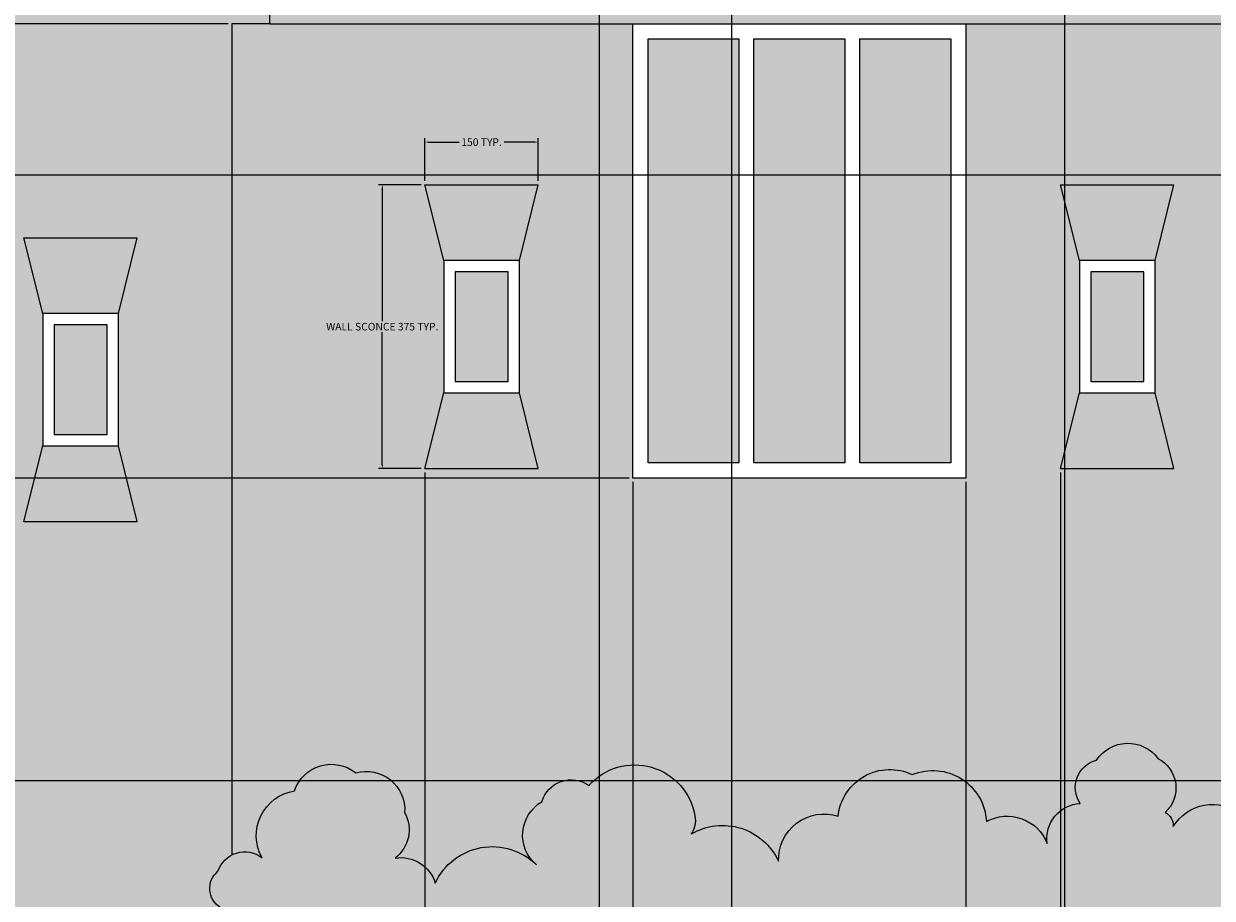
# Model space of a CAD drawing. Units: millimetres. Extents: x 2970 to 7764, y 2196 to 7505.
# Tile 3 of 13: x 4081 to 5651, y 3051 to 4206. Entities that reach past the tile are written whole.
import ezdxf

# ---------------------------------------------------------------- set-up
doc = ezdxf.new("R2010")
doc.units = ezdxf.units.MM
doc.header["$MEASUREMENT"] = 0
for name, color, linetype, lineweight in [('A-ANNO-DIMS', 2, 'Continuous', 18), ('A-ELEV', 7, 'Continuous', 25), ('A-ELEV-PATT', 8, 'Continuous', 13), ('A-GLAZ', 4, 'Continuous', 18), ('E-LITE', 2, 'Continuous', 18)]:
    doc.layers.add(name, color=color, linetype=linetype, lineweight=lineweight)
doc.styles.get("Standard").update_dxf_attribs({"font": 'arial.ttf'})
doc.dimstyles.get("Standard").update_dxf_attribs({"dimtxt": 10, "dimasz": 5, "dimexe": 5, "dimexo": 5, "dimgap": 2, "dimtad": 0, "dimtih": 1, "dimtoh": 1, "dimdec": 0, "dimzin": 0, "dimdsep": 46, "dimtxsty": 'Standard', "dimcen": 2, "dimadec": 0, "dimazin": 0, "dimtfac": 1, "dimtdec": 0, "dimtofl": 0, "dimtmove": 0, "dimatfit": 3, "dimfxl": 1, "dimtolj": 1, "dimtzin": 0, "dimarcsym": 0})

# ---------------------------------------------------------------- blocks, each defined once
blk = doc.blocks.new('WALL-SCONCE')
for p, q in [((4105.5, 5503.3), (4080.5, 5603.3)), ((4080.5, 5603.3), (4230.5, 5603.3)), ((4205.5, 5503.3), (4230.5, 5603.3)), ((4080.5, 5228.3), (4105.5, 5328.3)), ((4230.5, 5228.3), (4205.5, 5328.3)), ((4080.5, 5228.3), (4230.5, 5228.3))]:
    blk.add_line(p, q)
blk.add_lwpolyline([(4105.5, 5328.3), (4205.5, 5328.3), (4205.5, 5503.3), (4105.5, 5503.3)], close=True)
blk = doc.blocks.new('WIN-PANE')
blk.add_line((120, 560), (120, 0))
blk.add_lwpolyline([(120, 0), (0, 0), (0, 560), (120, 560)])
blk = doc.blocks.new('*D6')
at = {"layer": 'A-ANNO-DIMS', "color": 0, "lineweight": -2, "transparency": 16777216}
for p, q in [((4605.5, 3993.3), (4549.3, 3993.3)), ((4554.3, 3988.3), (4554.3, 3813)), ((4554.3, 3623.3), (4554.3, 3798.6)), ((4605.5, 3618.3), (4549.3, 3618.3))]:
    blk.add_line(p, q, dxfattribs=at)
at = {"layer": 'A-ANNO-DIMS', "color": 0, "transparency": 16777216}
for points in [[(4553.4, 3988.3), (4555.1, 3988.3), (4554.3, 3993.3)], [(4553.4, 3623.3), (4555.1, 3623.3), (4554.3, 3618.3)]]:
    blk.add_solid(points, dxfattribs=at)
at = {"layer": 'Defpoints', "color": 0, "transparency": 16777216}
for p in [(4554.3, 3993.3), (4610.5, 3993.3), (4610.5, 3618.3)]:
    blk.add_point(p, dxfattribs=at)
at = {"layer": 'A-ANNO-DIMS', "color": 0, "transparency": 16777216, "insert": (4554.3, 3805.8), "char_height": 10, "attachment_point": 5}
blk.add_mtext('\\A1;WALL SCONCE 375 TYP.', dxfattribs=at)
blk = doc.blocks.new('*D7')
at = {"layer": 'A-ANNO-DIMS', "color": 0, "lineweight": -2, "transparency": 16777216}
for p, q in [((4610.5, 3998.3), (4610.5, 4054.5)), ((4760.5, 3998.3), (4760.5, 4054.5)), ((4615.5, 4049.5), (4655.7, 4049.5)), ((4755.5, 4049.5), (4715.3, 4049.5))]:
    blk.add_line(p, q, dxfattribs=at)
at = {"layer": 'A-ANNO-DIMS', "color": 0, "transparency": 16777216}
for points in [[(4615.5, 4050.4), (4615.5, 4048.7), (4610.5, 4049.5)], [(4755.5, 4050.4), (4755.5, 4048.7), (4760.5, 4049.5)]]:
    blk.add_solid(points, dxfattribs=at)
at = {"layer": 'Defpoints', "color": 0, "transparency": 16777216}
for p in [(4760.5, 4049.5), (4610.5, 3993.3), (4760.5, 3993.3)]:
    blk.add_point(p, dxfattribs=at)
at = {"layer": 'A-ANNO-DIMS', "color": 0, "transparency": 16777216, "insert": (4685.5, 4049.5), "char_height": 10, "attachment_point": 5}
blk.add_mtext('\\A1;150 TYP.', dxfattribs=at)
blk = doc.blocks.new('*D45')
at = {"layer": 'A-ANNO-DIMS', "color": 0, "lineweight": -2, "transparency": 16777216}
for p, q in [((4880.5, 3605.8), (2982.5, 3605.8)), ((2987.5, 3600.8), (2987.5, 3307.9)), ((2987.5, 3000.8), (2987.5, 3293.7)), ((4350.5, 2995.8), (2982.5, 2995.8))]:
    blk.add_line(p, q, dxfattribs=at)
at = {"layer": 'A-ANNO-DIMS', "color": 0, "transparency": 16777216}
for points in [[(2986.7, 3600.8), (2988.3, 3600.8), (2987.5, 3605.8)], [(2986.7, 3000.8), (2988.3, 3000.8), (2987.5, 2995.8)]]:
    blk.add_solid(points, dxfattribs=at)
at = {"layer": 'Defpoints', "color": 0, "transparency": 16777216}
for p in [(2987.5, 3605.8), (4885.5, 3605.8), (4355.5, 2995.8)]:
    blk.add_point(p, dxfattribs=at)
at = {"layer": 'A-ANNO-DIMS', "color": 0, "transparency": 16777216, "insert": (2987.5, 3300.8), "char_height": 10, "attachment_point": 5}
blk.add_mtext('\\A1;610', dxfattribs=at)
blk = doc.blocks.new('*D46')
at = {"layer": 'A-ANNO-DIMS', "color": 0, "lineweight": -2, "transparency": 16777216}
for p, q in [((4350.5, 4205.8), (2982.5, 4205.8)), ((2987.5, 4200.8), (2987.5, 3912.9)), ((2987.5, 3610.8), (2987.5, 3898.7)), ((4880.5, 3605.8), (2982.5, 3605.8))]:
    blk.add_line(p, q, dxfattribs=at)
at = {"layer": 'A-ANNO-DIMS', "color": 0, "transparency": 16777216}
for points in [[(2986.7, 4200.8), (2988.3, 4200.8), (2987.5, 4205.8)], [(2986.7, 3610.8), (2988.3, 3610.8), (2987.5, 3605.8)]]:
    blk.add_solid(points, dxfattribs=at)
at = {"layer": 'Defpoints', "color": 0, "transparency": 16777216}
for p in [(2987.5, 4205.8), (4355.5, 4205.8), (4885.5, 3605.8)]:
    blk.add_point(p, dxfattribs=at)
at = {"layer": 'A-ANNO-DIMS', "color": 0, "transparency": 16777216, "insert": (2987.5, 3905.8), "char_height": 10, "attachment_point": 5}
blk.add_mtext('\\A1;600', dxfattribs=at)
blk = doc.blocks.new('*D47')
at = {"layer": 'A-ANNO-DIMS', "color": 0, "lineweight": -2, "transparency": 16777216}
for p, q in [((4610.5, 3613.3), (4610.5, 2197.8)), ((4885.5, 3600.8), (4885.5, 2197.8)), ((4615.5, 2202.8), (4734.8, 2202.8)), ((4880.5, 2202.8), (4761.2, 2202.8))]:
    blk.add_line(p, q, dxfattribs=at)
at = {"layer": 'A-ANNO-DIMS', "color": 0, "transparency": 16777216}
for points in [[(4615.5, 2203.6), (4615.5, 2202), (4610.5, 2202.8)], [(4880.5, 2203.6), (4880.5, 2202), (4885.5, 2202.8)]]:
    blk.add_solid(points, dxfattribs=at)
at = {"layer": 'Defpoints', "color": 0, "transparency": 16777216}
for p in [(4610.5, 3618.3), (4885.5, 3605.8), (4885.5, 2202.8)]:
    blk.add_point(p, dxfattribs=at)
at = {"layer": 'A-ANNO-DIMS', "color": 0, "transparency": 16777216, "insert": (4748, 2202.8), "char_height": 10, "attachment_point": 5}
blk.add_mtext('\\A1;275', dxfattribs=at)
blk = doc.blocks.new('*D48')
at = {"layer": 'A-ANNO-DIMS', "color": 0, "lineweight": -2, "transparency": 16777216}
for p, q in [((5450.5, 3613.3), (5450.5, 2197.8)), ((5325.5, 3600.8), (5325.5, 2197.8)), ((5330.5, 2202.8), (5375.4, 2202.8)), ((5445.5, 2202.8), (5400.6, 2202.8))]:
    blk.add_line(p, q, dxfattribs=at)
at = {"layer": 'A-ANNO-DIMS', "color": 0, "transparency": 16777216}
for points in [[(5330.5, 2203.6), (5330.5, 2202), (5325.5, 2202.8)], [(5445.5, 2203.6), (5445.5, 2202), (5450.5, 2202.8)]]:
    blk.add_solid(points, dxfattribs=at)
at = {"layer": 'Defpoints', "color": 0, "transparency": 16777216}
for p in [(5450.5, 3618.3), (5325.5, 3605.8), (5450.5, 2202.8)]:
    blk.add_point(p, dxfattribs=at)
at = {"layer": 'A-ANNO-DIMS', "color": 0, "transparency": 16777216, "insert": (5388, 2202.8), "char_height": 10, "attachment_point": 5}
blk.add_mtext('\\A1;125', dxfattribs=at)
blk = doc.blocks.new('*D49')
at = {"layer": 'A-ANNO-DIMS', "color": 0, "lineweight": -2, "transparency": 16777216}
for p, q in [((5950.3, 4005.8), (2982.5, 4005.8)), ((2987.5, 4000.8), (2987.5, 3612.9)), ((2987.5, 3210.8), (2987.5, 3598.7)), ((5950.3, 3205.8), (2982.5, 3205.8))]:
    blk.add_line(p, q, dxfattribs=at)
at = {"layer": 'A-ANNO-DIMS', "color": 0, "transparency": 16777216}
for points in [[(2986.7, 4000.8), (2988.3, 4000.8), (2987.5, 4005.8)], [(2986.7, 3210.8), (2988.3, 3210.8), (2987.5, 3205.8)]]:
    blk.add_solid(points, dxfattribs=at)
at = {"layer": 'Defpoints', "color": 0, "transparency": 16777216}
for p in [(2987.5, 4005.8), (5955.3, 4005.8), (5955.3, 3205.8)]:
    blk.add_point(p, dxfattribs=at)
at = {"layer": 'A-ANNO-DIMS', "color": 0, "transparency": 16777216, "insert": (2987.5, 3605.8), "char_height": 10, "attachment_point": 5}
blk.add_mtext('\\A1;800', dxfattribs=at)
blk = doc.blocks.new('*D56')
at = {"layer": 'A-ANNO-DIMS', "color": 0, "lineweight": -2, "transparency": 16777216}
for p, q in [((5015.8, 5457.5), (5015.8, 2197.8)), ((5455.8, 5457.5), (5455.8, 2197.8)), ((5020.8, 2202.8), (5222.6, 2202.8)), ((5450.8, 2202.8), (5249, 2202.8))]:
    blk.add_line(p, q, dxfattribs=at)
at = {"layer": 'A-ANNO-DIMS', "color": 0, "transparency": 16777216}
for points in [[(5020.8, 2203.6), (5020.8, 2202), (5015.8, 2202.8)], [(5450.8, 2203.6), (5450.8, 2202), (5455.8, 2202.8)]]:
    blk.add_solid(points, dxfattribs=at)
at = {"layer": 'Defpoints', "color": 0, "transparency": 16777216}
for p in [(5015.8, 5462.5), (5455.8, 5462.5), (5455.8, 2202.8)]:
    blk.add_point(p, dxfattribs=at)
at = {"layer": 'A-ANNO-DIMS', "color": 0, "transparency": 16777216, "insert": (5235.8, 2202.8), "char_height": 10, "attachment_point": 5}
blk.add_mtext('\\A1;440', dxfattribs=at)
blk = doc.blocks.new('*D57')
at = {"layer": 'A-ANNO-DIMS', "color": 0, "lineweight": -2, "transparency": 16777216}
for p, q in [((5455.8, 5457.5), (5455.8, 2197.8)), ((5755.5, 5000.8), (5755.5, 2197.8)), ((5460.8, 2202.8), (5586.7, 2202.8)), ((5750.5, 2202.8), (5624.6, 2202.8))]:
    blk.add_line(p, q, dxfattribs=at)
at = {"layer": 'A-ANNO-DIMS', "color": 0, "transparency": 16777216}
for points in [[(5460.8, 2203.6), (5460.8, 2202), (5455.8, 2202.8)], [(5750.5, 2203.6), (5750.5, 2202), (5755.5, 2202.8)]]:
    blk.add_solid(points, dxfattribs=at)
at = {"layer": 'Defpoints', "color": 0, "transparency": 16777216}
for p in [(5455.8, 5462.5), (5755.5, 5005.8), (5755.5, 2202.8)]:
    blk.add_point(p, dxfattribs=at)
at = {"layer": 'A-ANNO-DIMS', "color": 0, "transparency": 16777216, "insert": (5605.7, 2202.8), "char_height": 10, "attachment_point": 5}
blk.add_mtext('\\A1;299.7', dxfattribs=at)
blk = doc.blocks.new('*D66')
at = {"layer": 'A-ANNO-DIMS', "color": 0, "lineweight": -2, "transparency": 16777216}
for p, q in [((4840.8, 6232.5), (4840.8, 2197.8)), ((5015.8, 6057.5), (5015.8, 2197.8)), ((4845.8, 2202.8), (4915.7, 2202.8)), ((5010.8, 2202.8), (4940.9, 2202.8))]:
    blk.add_line(p, q, dxfattribs=at)
at = {"layer": 'A-ANNO-DIMS', "color": 0, "transparency": 16777216}
for points in [[(4845.8, 2203.6), (4845.8, 2202), (4840.8, 2202.8)], [(5010.8, 2203.6), (5010.8, 2202), (5015.8, 2202.8)]]:
    blk.add_solid(points, dxfattribs=at)
at = {"layer": 'Defpoints', "color": 0, "transparency": 16777216}
for p in [(4840.8, 6237.5), (5015.8, 6062.5), (5015.8, 2202.8)]:
    blk.add_point(p, dxfattribs=at)
at = {"layer": 'A-ANNO-DIMS', "color": 0, "transparency": 16777216, "insert": (4928.3, 2202.8), "char_height": 10, "attachment_point": 5}
blk.add_mtext('\\A1;175', dxfattribs=at)

msp = doc.modelspace()

# ---------------------------------------------------------------- hatches: boundary and pattern name
at = {"layer": 'A-ELEV-PATT'}
h = msp.add_hatch(color=256, dxfattribs=at)
h.dxf.hatch_style = 1
h.paths.add_polyline_path([(6405.5, 7255.789), (4305.5, 7255.789), (4305.5, 6505.789), (3730.5, 6505.789), (3730.5, 4205.789), (3730.5, 2945.789), (3730.5, 2895.789), (3830.5, 2895.789), (3830.5, 4205.789), (3830.5, 6405.789), (4405.5, 6405.789), (4405.5, 4205.789), (6905.5, 4205.789), (6905.5, 2945.789), (6905.5, 2845.789), (7155.5, 2845.789), (7155.5, 2945.789), (7155.5, 4205.789), (7155.5, 4455.789), (4555.5, 4455.789), (4555.5, 6505.789), (4555.5, 7005.789), (6155.5, 7005.789), (6155.5, 6755.789), (6405.5, 6755.789)])
h.paths.add_polyline_path([(7405.5, 6755.789), (6155.5, 6755.789), (5755.5, 6755.789), (5755.5, 5005.789), (7405.5, 5005.789)])
h.paths.add_polyline_path([(7155.5, 6505.789), (7155.5, 5255.789), (6005.5, 5255.789), (6005.5, 6505.789)], flags=16)
h.paths.add_polyline_path([(6105.5, 5520.789), (6105.5, 6055.789), (6455.5, 6055.789), (6455.5, 5520.789), (6655.5, 5520.789), (6655.5, 5605.789), (6655.5, 5955.789), (6955.5, 5955.789), (6955.5, 5605.789), (6955.5, 5520.789)], flags=0)
h.paths.add_polyline_path([(6425.5, 5755.789), (6425.5, 5655.789), (6425.5, 5555.789), (6405.5, 5555.789), (6405.5, 5755.789)], flags=0)
h.paths.add_polyline_path([(6955.5, 5505.789), (6955.5, 5405.789), (6655.5, 5405.789), (6655.5, 5505.789)], flags=0)
h = msp.add_hatch(color=256, dxfattribs=at)
h.set_gradient(color1=(53, 53, 54), color2=(99, 100, 102), name='SPHERICAL')
h.paths.add_polyline_path([(4405.5, 6255.789), (3905.5, 6255.789), (3905.5, 4205.789), (3905.5, 2895.789), (4355.5, 2895.789), (4355.5, 2995.799, -0.50803883), (4340.162, 3038.75, -0.52056705), (4337.177, 3086.472, -0.19797947), (4355.5, 3108.072), (4355.5, 4205.789), (4405.5, 4205.789)])
h.paths.add_polyline_path([(4080.5, 5228.289), (4105.5, 5328.289), (4105.5, 5503.289), (4080.5, 5603.289), (4230.5, 5603.289), (4205.5, 5503.289), (4205.5, 5328.289), (4230.5, 5228.289)], flags=16)
h.paths.add_polyline_path([(4120.5, 5343.289), (4120.5, 5488.289), (4190.5, 5488.289), (4190.5, 5343.289)], flags=0)
h.paths.add_polyline_path([(4230.5, 3923.289), (4205.5, 3823.289), (4205.5, 3648.289), (4230.5, 3548.289), (4080.5, 3548.289), (4105.5, 3648.289), (4105.5, 3823.289), (4080.5, 3923.289)], flags=16)
h.paths.add_polyline_path([(4190.5, 3808.289), (4190.5, 3663.289), (4120.5, 3663.289), (4120.5, 3808.289)], flags=0)
h = msp.add_hatch(color=256, dxfattribs=at)
h.set_gradient(color1=(248, 215, 49), color2=(241, 235, 31), name='INVCYLINDER')
h.paths.add_polyline_path([(5490.5, 3733.289), (5560.5, 3733.289), (5560.5, 3878.289), (5490.5, 3878.289)])
h.paths.add_polyline_path([(4720.5, 3878.289), (4650.5, 3878.289), (4650.5, 3733.289), (4720.5, 3733.289)])
h.paths.add_polyline_path([(4120.5, 3663.289), (4190.5, 3663.289), (4190.5, 3808.289), (4120.5, 3808.289)])
h.paths.add_polyline_path([(4190.5, 5488.289), (4120.5, 5488.289), (4120.5, 5343.289), (4190.5, 5343.289)])
h = msp.add_hatch(color=256, dxfattribs=at)
h.set_gradient(color1=(199, 200, 202), color2=(147, 149, 152), name='INVSPHERICAL')
h.paths.add_polyline_path([(5254.666, 3214.122, -0.52056705), (5352.552, 3152.098, -0.4540886), (5432.911, 3123.272, -0.43983375), (5476.699, 3175.953, -0.52056705), (5498.186, 3233.206, -0.52056705), (5579.359, 3235.592, -0.52056705), (5588.909, 3164.025, -0.30236269), (5599.555, 3145.665, -0.44962196), (5689.182, 3161.64, -0.52056705), (5705.894, 3233.206, -0.52056705), (5748.868, 3259.448, -0.32013944), (5784.015, 3210.89, -0.25799727), (5820.491, 3221.279, -0.38376587), (5855.271, 3235.313), (5855.271, 4205.789), (5325.5, 4205.789), (5325.5, 3605.789), (4885.5, 3605.789), (4885.5, 4205.789), (4405.5, 4205.789), (4355.5, 4205.789), (4355.5, 3108.072, -0.29244748), (4395.384, 3104.368, -0.52056705), (4438.16, 3192.652, -0.52056705), (4519.333, 3216.508, -0.52056705), (4583.794, 3164.025, -0.37342356), (4571.284, 3103.834, -0.37512524), (4624.381, 3070.989, -0.49967099), (4754.056, 3098.592, -0.48686678), (4765.24, 3178.339, -0.52056705), (4827.314, 3199.809, -0.63134555), (4967.523, 3159.254, -0.19603193), (4962.635, 3135.756, -0.44420267), (5077.995, 3099.615, -0.52056705), (5156.781, 3159.254, -0.52056705)])
h.paths.add_polyline_path([(5450.5, 3618.289), (5475.5, 3718.289), (5475.5, 3893.289), (5450.5, 3993.289), (5600.5, 3993.289), (5575.5, 3893.289), (5575.5, 3718.289), (5600.5, 3618.289)], flags=16)
h.paths.add_polyline_path([(5490.5, 3733.289), (5490.5, 3878.289), (5560.5, 3878.289), (5560.5, 3733.289)], flags=0)
h.paths.add_polyline_path([(4760.5, 3618.289), (4610.5, 3618.289), (4635.5, 3718.289), (4635.5, 3893.289), (4610.5, 3993.289), (4760.5, 3993.289), (4735.5, 3893.289), (4735.5, 3718.289)], flags=16)
h.paths.add_polyline_path([(4720.5, 3733.289), (4650.5, 3733.289), (4650.5, 3878.289), (4720.5, 3878.289)], flags=0)
h = msp.add_hatch(color=256, dxfattribs=at)
h.set_gradient(color1=(122, 175, 223), color2=(173, 221, 247), name='SPHERICAL')
h.paths.add_polyline_path([(4905.5, 3625.789), (5025.5, 3625.789), (5025.5, 4185.789), (4905.5, 4185.789)])
h.paths.add_polyline_path([(5045.5, 3625.789), (5165.5, 3625.789), (5165.5, 4185.789), (5045.5, 4185.789)])
h.paths.add_polyline_path([(5305.5, 4185.789), (5185.5, 4185.789), (5185.5, 3625.789), (5305.5, 3625.789)])
h = msp.add_hatch(color=256, dxfattribs=at)
h.set_gradient(color1=(248, 215, 49), color2=(199, 200, 202), name='INVHEMISPHERICAL')
h.paths.add_polyline_path([(4610.5, 3993.289), (4635.5, 3893.289), (4735.5, 3893.289), (4760.5, 3993.289)])
h = msp.add_hatch(color=256, dxfattribs=at)
h.set_gradient(color1=(248, 215, 49), color2=(199, 200, 202), name='INVHEMISPHERICAL')
h.paths.add_polyline_path([(5450.5, 3993.289), (5475.5, 3893.289), (5575.5, 3893.289), (5600.5, 3993.289)])
h = msp.add_hatch(color=256, dxfattribs=at)
h.set_gradient(color1=(241, 235, 31), color2=(99, 100, 102), name='INVCURVED')
h.paths.add_polyline_path([(4205.5, 3823.289), (4230.5, 3923.289), (4080.5, 3923.289), (4105.5, 3823.289)])
h = msp.add_hatch(color=256, dxfattribs=at)
h.set_gradient(color1=(248, 215, 49), color2=(199, 200, 202), name='HEMISPHERICAL')
h.paths.add_polyline_path([(4760.5, 3618.289), (4735.5, 3718.289), (4635.5, 3718.289), (4610.5, 3618.289)])
h = msp.add_hatch(color=256, dxfattribs=at)
h.set_gradient(color1=(248, 215, 49), color2=(199, 200, 202), name='HEMISPHERICAL')
h.paths.add_polyline_path([(5600.5, 3618.289), (5575.5, 3718.289), (5475.5, 3718.289), (5450.5, 3618.289)])
h = msp.add_hatch(color=256, dxfattribs=at)
h.set_gradient(color1=(241, 235, 31), color2=(99, 100, 102), name='CURVED')
h.paths.add_polyline_path([(4230.5, 3548.289), (4205.5, 3648.289), (4105.5, 3648.289), (4080.5, 3548.289)])
h = msp.add_hatch(color=256, dxfattribs=at)
h.set_gradient(color1=(0, 255, 0), color2=(0, 153, 0), name='INVCURVED')
h.paths.add_polyline_path([(5156.781, 3159.254, 0.52056705), (5077.995, 3099.615, 0.44420267), (4962.635, 3135.756, 0.17969754), (4967.824, 3157.271, 0.6400553), (4827.314, 3199.809, 0.52056705), (4765.24, 3178.339, 0.48686678), (4754.056, 3098.592, -0.0165827), (4758.078, 3094.844, -0.02688608), (4754.056, 3098.592, 0.49967099), (4624.381, 3070.989, 0.37512524), (4571.284, 3103.834, 0.37342356), (4583.794, 3164.025, 0.52056705), (4519.333, 3216.508, 0.52056705), (4438.16, 3192.652, 0.52056705), (4395.384, 3104.368, 0.52056705), (4337.177, 3086.472, 0.52056705), (4340.162, 3038.75, 0.50842605), (4355.534, 2995.789), (5854.747, 2995.789, 0.43666624), (5849.141, 3020.892, 0.52056705), (5873.015, 3051.904, 0.52056705), (5873.015, 3123.471, 0.52056705), (5877.79, 3197.423, 0.52056705), (5865.853, 3228.435, 0.52056705), (5820.491, 3221.279, 0.25799727), (5784.015, 3210.89, 0.32013944), (5748.868, 3259.448, 0.52056705), (5705.894, 3233.206, 0.52056705), (5689.182, 3161.64, 0.44962196), (5599.555, 3145.665, 0.30236269), (5588.909, 3164.025, 0.52056705), (5579.359, 3235.592, 0.52056705), (5498.186, 3233.206, 0.52056705), (5476.699, 3175.953, 0.43983375), (5432.911, 3123.272, 0.4540886), (5352.552, 3152.098, 0.52056705), (5254.666, 3214.122, 0.52056705)])

# ---------------------------------------------------------------- linework, layer by layer
at = {"layer": 'A-ELEV'}
for p, q in [((4405.5, 4205.789), (4405.5, 6405.789)), ((4405.5, 4205.789), (4355.5, 4205.789)), ((4355.5, 4205.789), (4355.5, 3108.072)), ((4405.5, 4205.789), (6905.5, 4205.789)), ((4885.5, 4205.789), (5325.5, 4205.789)), ((4885.5, 3605.789), (4885.5, 4205.789)), ((5325.5, 4205.789), (5325.5, 3605.789)), ((5325.5, 3605.789), (4885.5, 3605.789))]:
    msp.add_line(p, q, dxfattribs=at)
for points in [[(4650.5, 3733.289), (4720.5, 3733.289), (4720.5, 3878.289), (4650.5, 3878.289)], [(5490.5, 3733.289), (5560.5, 3733.289), (5560.5, 3878.289), (5490.5, 3878.289)], [(4120.5, 3663.289), (4190.5, 3663.289), (4190.5, 3808.289), (4120.5, 3808.289)]]:
    msp.add_lwpolyline(points, close=True, dxfattribs=at)
for points in [[(5432.911, 3123.272, -0.43983375), (5476.699, 3175.953, -0.52056705), (5498.186, 3233.206, -0.52056705), (5579.359, 3235.592, -0.52056705), (5588.909, 3164.025, -0.30236269), (5599.555, 3145.665)], [(5599.555, 3145.665, -0.44962196), (5689.182, 3161.64, -0.52056705), (5705.894, 3233.206, -0.52056705), (5748.868, 3259.448, -0.32013944), (5784.015, 3210.89)], [(4355.534, 2995.789, -0.50842605), (4340.162, 3038.75, -0.52056705), (4337.177, 3086.472, -0.52056705), (4395.384, 3104.368, -0.52056705), (4438.16, 3192.652, -0.52056705), (4519.333, 3216.508, -0.52056705), (4583.794, 3164.025, -0.37342356), (4571.284, 3103.834, -0.37342356)], [(4571.284, 3103.834, -0.37512524), (4624.381, 3070.989, -0.52056705), (4758.078, 3094.844, -0.52056705), (4765.24, 3178.339, -0.52056705), (4827.314, 3199.809, -0.63134555), (4967.523, 3159.254, -0.19603193), (4962.635, 3135.756)], [(4962.635, 3135.756, -0.44420267), (5077.995, 3099.615, -0.52056705), (5156.781, 3159.254, -0.52056705), (5254.666, 3214.122, -0.52056705), (5352.552, 3152.098, -0.4540886), (5432.911, 3123.272, -0.4540886)]]:
    msp.add_lwpolyline(points, format="xyb", dxfattribs=at)

# ---------------------------------------------------------------- block references
at = {"layer": 'A-GLAZ'}
msp.add_blockref('WIN-PANE', (4905.5, 3625.789), dxfattribs=at)
at = {"layer": 'A-GLAZ', "rotation": 180}
for p in [(5165.5, 4185.789), (5305.5, 4185.789)]:
    msp.add_blockref('WIN-PANE', p, dxfattribs=at)
at = {"layer": 'E-LITE'}
for p in [(530, -1610), (1370, -1610), (0, -1680)]:
    msp.add_blockref('WALL-SCONCE', p, dxfattribs=at)

# ---------------------------------------------------------------- dimensions: what is measured, and where the dimension line sits
at = {"layer": 'A-ANNO-DIMS'}
for base, p1, p2, override, picture, middle in [((5015.81, 2202.789), (4840.81, 6237.49), (5015.81, 6062.49), {"dimdec": 0, "dimlfac": 1, "dimrnd": 0, "dimzin": 0, "dimdsep": 46, "dimlunit": 2}, '*D66', (4928.31, 2202.789)), ((5455.81, 2202.789), (5015.81, 5462.49), (5455.81, 5462.49), {"dimdec": 0, "dimlfac": 1, "dimrnd": 0, "dimzin": 0, "dimdsep": 46, "dimlunit": 2}, '*D56', (5235.81, 2202.789)), ((5755.5, 2202.789), (5455.81, 5462.49), (5755.5, 5005.789), {"dimdec": 1, "dimlfac": 1, "dimrnd": 0, "dimzin": 0, "dimdsep": 46, "dimlunit": 2}, '*D57', (5605.655, 2202.789)), ((4885.5, 2202.789), (4610.5, 3618.289), (4885.5, 3605.789), {"dimdec": 0, "dimlfac": 1, "dimrnd": 0, "dimzin": 0, "dimdsep": 46, "dimlunit": 2}, '*D47', (4748, 2202.789)), ((5450.5, 2202.789), (5325.5, 3605.789), (5450.5, 3618.289), {"dimdec": 0, "dimlfac": 1, "dimrnd": 0, "dimzin": 0, "dimdsep": 46, "dimlunit": 2}, '*D48', (5388, 2202.789))]:
    dim = msp.add_linear_dim(base=base, p1=p1, p2=p2, dimstyle='Standard', override=override, dxfattribs=at)
    dim.commit()
    dim.dimension.update_dxf_attribs({"geometry": picture, "text_midpoint": middle})
for base, p1, p2, picture, middle in [((2987.5, 4205.789), (4885.5, 3605.789), (4355.5, 4205.789), '*D46', (2987.5, 3905.789)), ((2987.5, 4005.789), (5955.271, 3205.789), (5955.271, 4005.789), '*D49', (2987.5, 3605.789)), ((2987.5, 3605.789), (4355.5, 2995.789), (4885.5, 3605.789), '*D45', (2987.5, 3300.789))]:
    dim = msp.add_linear_dim(base=base, p1=p1, p2=p2, angle=90, dimstyle='Standard', override={"dimdec": 0, "dimlfac": 1, "dimrnd": 0, "dimzin": 0, "dimdsep": 46, "dimlunit": 2}, dxfattribs=at)
    dim.commit()
    dim.dimension.update_dxf_attribs({"geometry": picture, "text_midpoint": middle})
dim = msp.add_linear_dim(base=(4760.5, 4049.539), p1=(4610.5, 3993.289), p2=(4760.5, 3993.289), text='<> TYP.', dimstyle='Standard', override={"dimdec": 0, "dimlfac": 1, "dimrnd": 0, "dimzin": 0, "dimdsep": 46, "dimlunit": 2}, dxfattribs=at)
dim.commit()
dim.dimension.update_dxf_attribs({"geometry": '*D7', "text_midpoint": (4685.5, 4049.539)})
dim = msp.add_linear_dim(base=(4554.25, 3993.289), p1=(4610.5, 3618.289), p2=(4610.5, 3993.289), angle=90, text='WALL SCONCE <> TYP.', dimstyle='Standard', override={"dimdec": 0, "dimlfac": 1, "dimrnd": 0, "dimzin": 0, "dimdsep": 46, "dimlunit": 2}, dxfattribs=at)
dim.commit()
dim.dimension.update_dxf_attribs({"geometry": '*D6', "text_midpoint": (4554.25, 3805.789)})

doc.saveas('drawing.dxf')
